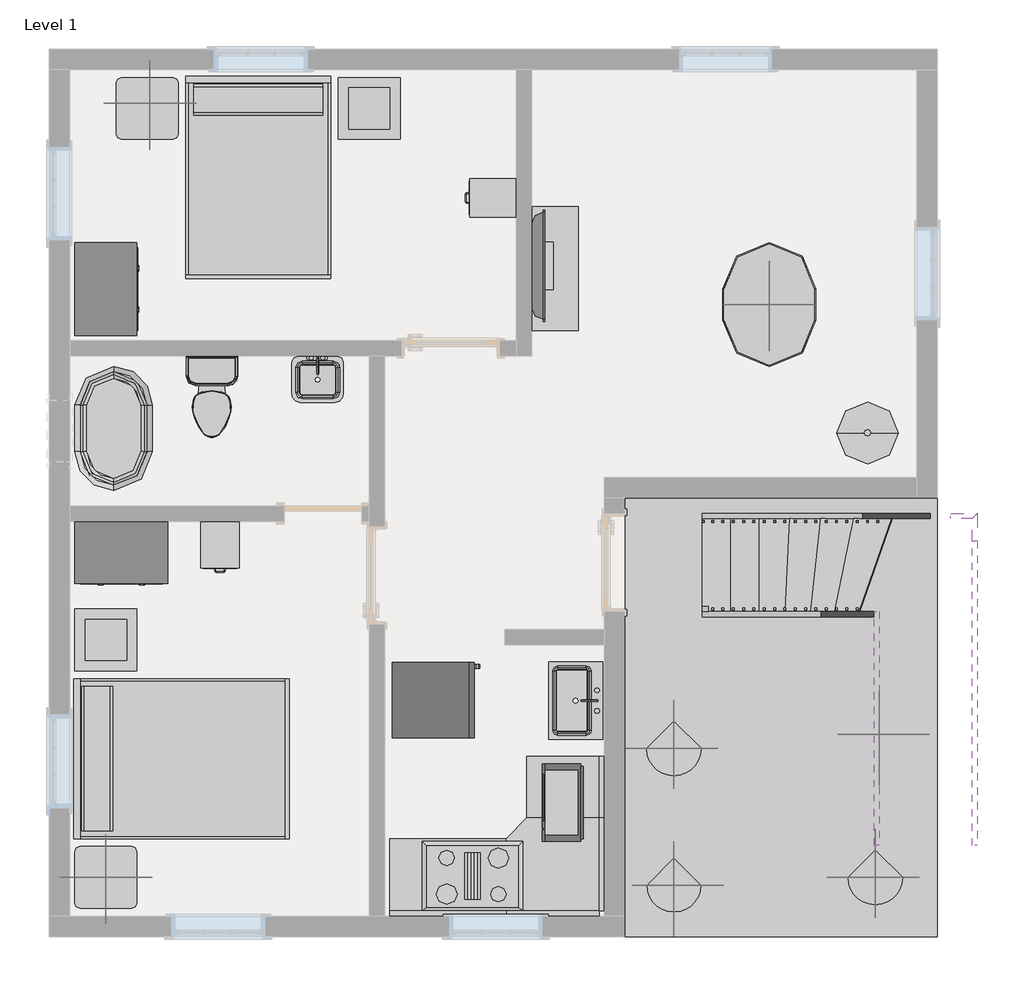
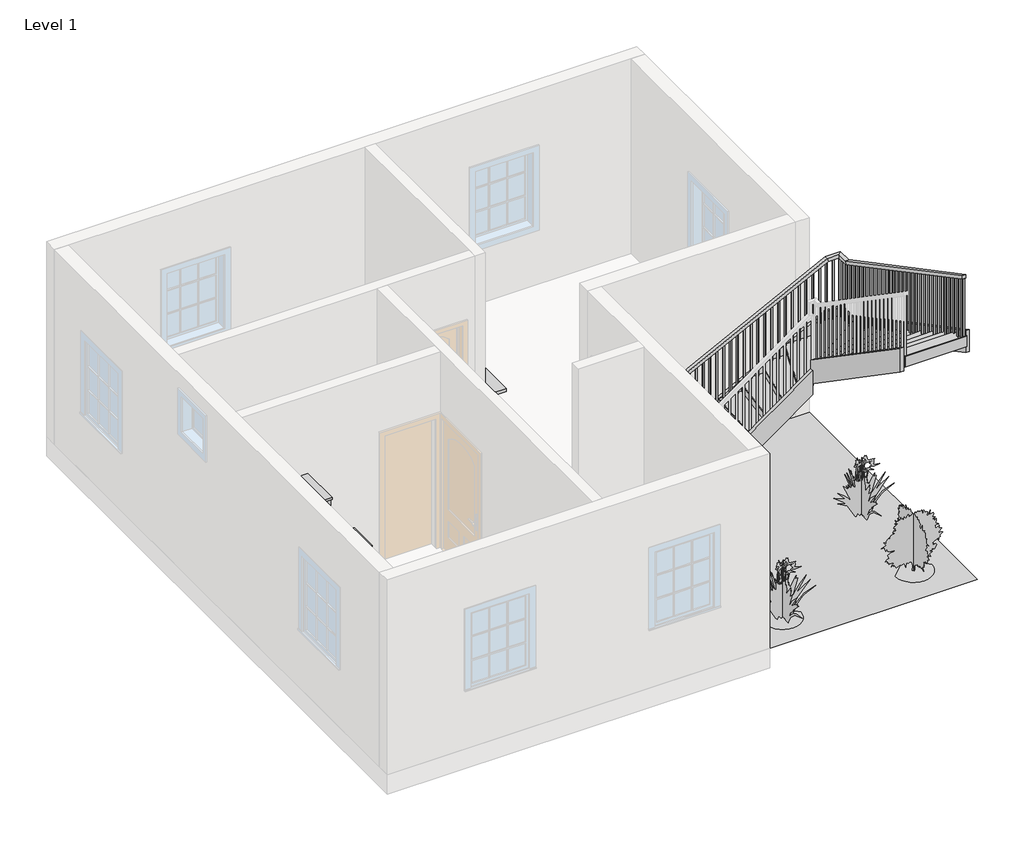
# One storey, part 2 of 2: 15 furniture elements, 7 geographic elements, 6 members, 5 flow terminals, 4 proxies, 1 railing, 1 stair flight.
"""IFC4 building model written with IfcOpenShell, lengths in millimetres."""

from ifc_helpers import new_model, si_unit, frame, origin, place, context, project, spatial, polyline, outline, extrude, faceted_brep, triangles, transform, mapped, element, save
from components import proxy_bb1e6e30, proxy_8a8d5ab2, proxy_a13a33b2, flow_terminal_accce45a, flow_terminal_38af2918, flow_terminal_62a433f7, toilet_domestic_3d_toilet_domestic_3d_f7549cf7, toilet_domestic_3d_toilet_domestic_3d_183bbd19, flow_terminal_04541809, furniture_096e7f55, furniture_35c09872, furniture_bb55ed6b, furniture_33655958, furniture_7a3aaa4f, furniture_b5c51a22, furniture_be1c6672, furniture_31d08a24, furniture_c21ab0ed, furniture_3250926c, furniture_e2d07697, rpc_plant_tropical_55f6ff97, rpc_plant_tropical_agave_1_5_93a2a214, rpc_plant_tropical_jungle_flame_3_9c4808c2, stair_flight_bb54b32b

model = new_model("IFC4")

# Units and contexts
model_context = context("Model", 3, world=origin())
ifc_project = project(units=[si_unit("LENGTHUNIT", "METRE", prefix="MILLI")], contexts=[model_context])

# Site, building, storey
site = spatial("IfcSite", under=ifc_project)
building = spatial("IfcBuilding", under=site)
storey = spatial("IfcBuildingStorey", under=building, Name="Level 1", Elevation=0.0)

# Proxies
placement = place(None, origin())
element("IfcBuildingElementProxy", 1, Name="Building Element Proxy", at=placement, inside=storey, context=model_context, shape_type="Tessellation", body=[
    triangles([(-7688.07724, 10762.3523804, 0.0), (-7688.07724, 6444.3525742, 0.0), (-4614.6770462, 6444.3525742, 0.0), (-4614.6770462, 10762.3523804, 0.0), (-7789.6768524, 6444.3525742, 0.0), (-7910.2003098, 6444.3525742, 0.0)], [[6, 5, 1], [2, 4, 1], [1, 5, 2], [2, 3, 4]], closed=False),
])
proxy_shape = proxy_bb1e6e30(model_context)
element("IfcBuildingElementProxy", 2, Name="Cook Top-4 Unit : 36\" x 20\"", ObjectType="Cook Top-4 Unit : 36\" x 20\"", at=placement, inside=storey, context=model_context, shape_type="MappedRepresentation", body=[
    mapped(proxy_shape, transform((-9186.6770189, 7041.2523405, 0.0), x_axis=(1.0, 0.0, 0.0), y_axis=(0.0, 1.0, 0.0), z_axis=(0.0, 0.0, 1.0))),
])
proxy_2_shape = proxy_8a8d5ab2(model_context)
element("IfcBuildingElementProxy", 3, Name="Microwave : 30\" x 16\" x 18\"", ObjectType="Microwave : 30\" x 16\" x 18\"", at=placement, inside=storey, context=model_context, shape_type="MappedRepresentation", body=[
    mapped(proxy_2_shape, transform((-7944.5965131, 8265.4452178, 0.0), x_axis=(0.0, -1.0000000000000002, 0.0), y_axis=(1.0000000000000002, 0.0, 0.0), z_axis=(0.0, 0.0, 1.0))),
])
proxy_3_shape = proxy_a13a33b2(model_context)
element("IfcBuildingElementProxy", 4, Name="Refrigerator : 30\" x 32\" RH", ObjectType="Refrigerator : 30\" x 32\" RH", at=placement, inside=storey, context=model_context, shape_type="MappedRepresentation", body=[
    mapped(proxy_3_shape, transform((-9585.5280474, 8773.2148405, 0.0), x_axis=(0.0, 1.0, 0.0), y_axis=(-1.0, 0.0, 0.0), z_axis=(0.0, 0.0, 1.0))),
])

# Flow terminals
flow_terminal_shape = flow_terminal_accce45a(model_context)
element("IfcFlowTerminal", 5, ObjectType="Floor Drain - Round : 5\" Strainer - 2\" Drain", at=placement, inside=storey, context=model_context, shape_type="MappedRepresentation", body=[
    mapped(flow_terminal_shape, transform((-12031.4770189, 10965.5523405, 0.0), x_axis=(1.0, 0.0, 0.0), y_axis=(0.0, 1.0, 0.0), z_axis=(0.0, 0.0, 1.0))),
])
flow_terminal_2_shape = flow_terminal_38af2918(model_context)
element("IfcFlowTerminal", 6, ObjectType="Sink Kitchen-Single : 30\" x 21\"", at=placement, inside=storey, context=model_context, shape_type="MappedRepresentation", body=[
    mapped(flow_terminal_2_shape, transform((-8173.02242, 8784.1415811, 0.0), x_axis=(0.0, -1.0000000000000004, 0.0), y_axis=(1.0000000000000004, 0.0, 0.0), z_axis=(0.0, 0.0, 1.0))),
])
flow_terminal_3_shape = flow_terminal_62a433f7(model_context)
element("IfcFlowTerminal", 7, ObjectType="Sink Vanity-Square : 20\" x 18\"", at=placement, inside=storey, context=model_context, shape_type="MappedRepresentation", body=[
    mapped(flow_terminal_3_shape, transform((-10726.3662595, 11979.2069394, 0.0), x_axis=(1.0, 0.0, 0.0), y_axis=(0.0, 1.0, 0.0), z_axis=(0.0, 0.0, 1.0))),
])
toilet_domestic_3d_toilet_domestic_3d_shape = toilet_domestic_3d_toilet_domestic_3d_f7549cf7(model_context)
toilet_domestic_3d_toilet_domestic_3d_2_shape = toilet_domestic_3d_toilet_domestic_3d_183bbd19(model_context)
element("IfcFlowTerminal", 8, ObjectType="Toilet-Domestic-3D : Toilet-Domestic-3D", at=placement, inside=storey, context=model_context, shape_type="MappedRepresentation", body=[
    mapped(toilet_domestic_3d_toilet_domestic_3d_shape, transform((-11752.0770189, 11664.6563132, 0.0), x_axis=(1.0, 0.0, 0.0), y_axis=(0.0, 1.0, 0.0), z_axis=(0.0, 0.0, 1.0))),
    mapped(toilet_domestic_3d_toilet_domestic_3d_2_shape, transform((-11752.0770189, 11664.6563132, 0.0), x_axis=(1.0, 0.0, 0.0), y_axis=(0.0, 1.0, 0.0), z_axis=(0.0, 0.0, 1.0))),
])
flow_terminal_4_shape = flow_terminal_04541809(model_context)
element("IfcFlowTerminal", 9, ObjectType="Tub-Free Standing-3D : 30\" x 60\"", at=placement, inside=storey, context=model_context, shape_type="MappedRepresentation", body=[
    mapped(flow_terminal_4_shape, transform((-12717.2770189, 11448.1523405, 0.0), x_axis=(1.0000000000000007, 0.0, 0.0), y_axis=(0.0, 1.0000000000000007, 0.0), z_axis=(0.0, 0.0, 1.0))),
])

# Furniture
furniture_shape = furniture_096e7f55(model_context)
element("IfcFurniture", 10, ObjectType="Bed-Shaker : Double 56\" x 78\"", at=placement, inside=storey, context=model_context, shape_type="MappedRepresentation", body=[
    mapped(furniture_shape, transform((-11275.8270189, 14902.5523405, 0.0), x_axis=(1.0, 0.0, 0.0), y_axis=(0.0, 1.0, 0.0), z_axis=(0.0, 0.0, 1.0))),
])
furniture_2_shape = furniture_35c09872(model_context)
element("IfcFurniture", 11, ObjectType="Bed-Shaker : Queen 62\" x 83\"", at=placement, inside=storey, context=model_context, shape_type="MappedRepresentation", body=[
    mapped(furniture_2_shape, transform((-13098.2770189, 8216.0023405, 0.0), x_axis=(0.0, 1.0, 0.0), y_axis=(-1.0, 0.0, 0.0), z_axis=(0.0, 0.0, 1.0))),
])
furniture_3_shape = furniture_bb55ed6b(model_context)
element("IfcFurniture", 12, ObjectType="Cabinet-File 2 Drawer : 15\" x 18\"", at=placement, inside=storey, context=model_context, shape_type="MappedRepresentation", body=[
    mapped(furniture_3_shape, transform((-8841.3427188, 13588.3042775, 0.0), x_axis=(0.0, -1.0000000000000004, 0.0), y_axis=(1.0000000000000004, 0.0, 0.0), z_axis=(0.0, 0.0, 1.0))),
])
element("IfcFurniture", 13, ObjectType="Cabinet-File 2 Drawer : 15\" x 18\"", at=placement, inside=storey, context=model_context, shape_type="MappedRepresentation", body=[
    mapped(furniture_3_shape, transform((-11543.5637717, 10447.2866406, 0.0), x_axis=(1.0, 0.0, 0.0), y_axis=(0.0, 1.0, 0.0), z_axis=(0.0, 0.0, 1.0))),
])
furniture_4_shape = furniture_33655958(model_context)
element("IfcFurniture", 14, ObjectType="Dresser : 48\" x 72\" x 24\"", at=placement, inside=storey, context=model_context, shape_type="MappedRepresentation", body=[
    mapped(furniture_4_shape, transform((-13156.639973, 13088.9456003, 0.0), x_axis=(0.0, 1.0000000000000002, 0.0), y_axis=(-1.0000000000000002, 0.0, 0.0), z_axis=(0.0, 0.0, 1.0))),
])
element("IfcFurniture", 15, ObjectType="Dresser : 48\" x 72\" x 24\"", at=placement, inside=storey, context=model_context, shape_type="MappedRepresentation", body=[
    mapped(furniture_4_shape, transform((-12371.8837591, 10592.1152946, 0.0), x_axis=(1.0, 0.0, 0.0), y_axis=(0.0, 1.0, 0.0), z_axis=(0.0, 0.0, 1.0))),
])
furniture_5_shape = furniture_7a3aaa4f(model_context)
element("IfcFurniture", 16, ObjectType="TV - Flat Screen : 42\"", at=placement, inside=storey, context=model_context, shape_type="MappedRepresentation", body=[
    mapped(furniture_5_shape, transform((-8543.9383953, 13052.2968547, 1041.4), x_axis=(0.0, 1.0, 0.0), y_axis=(-1.0, 0.0, 0.0), z_axis=(0.0, 0.0, 1.0))),
])
furniture_6_shape = furniture_b5c51a22(model_context)
element("IfcFurniture", 17, ObjectType="Table-Coffee : 24\" x 24\" x 24\"", at=placement, inside=storey, context=model_context, shape_type="MappedRepresentation", body=[
    mapped(furniture_6_shape, transform((-10220.9427856, 14502.5412627, 0.0), x_axis=(1.0, 0.0, 0.0), y_axis=(0.0, 1.0, 0.0), z_axis=(0.0, 0.0, 1.0))),
])
element("IfcFurniture", 18, ObjectType="Table-Coffee : 24\" x 24\" x 24\"", at=placement, inside=storey, context=model_context, shape_type="MappedRepresentation", body=[
    mapped(furniture_6_shape, transform((-12811.7427856, 9270.1412627, 0.0), x_axis=(1.0, 0.0, 0.0), y_axis=(0.0, 1.0, 0.0), z_axis=(0.0, 0.0, 1.0))),
])
furniture_7_shape = furniture_be1c6672(model_context)
element("IfcFurniture", 19, ObjectType="Table-Dining Oval : 36\" x 48\"", at=placement, inside=storey, context=model_context, shape_type="MappedRepresentation", body=[
    mapped(furniture_7_shape, transform((-6623.7753796, 13069.1720126, 0.0), x_axis=(0.0, 1.0, 0.0), y_axis=(-1.0, 0.0, 0.0), z_axis=(0.0, 0.0, 1.0))),
])
furniture_8_shape = furniture_31d08a24(model_context)
element("IfcFurniture", 20, ObjectType="Table-End : 24\" x 24\"", at=placement, inside=storey, context=model_context, shape_type="MappedRepresentation", body=[
    mapped(furniture_8_shape, transform((-12695.6106492, 14445.3523405, 0.0), x_axis=(1.0, 0.0, 0.0), y_axis=(0.0, 1.0, 0.0), z_axis=(0.0, 0.0, 1.0))),
])
element("IfcFurniture", 21, ObjectType="Table-End : 24\" x 24\"", at=placement, inside=storey, context=model_context, shape_type="MappedRepresentation", body=[
    mapped(furniture_8_shape, transform((-13102.0106492, 6876.1523405, 0.0), x_axis=(1.0, 0.0, 0.0), y_axis=(0.0, 1.0, 0.0), z_axis=(0.0, 0.0, 1.0))),
])
furniture_9_shape = furniture_c21ab0ed(model_context)
element("IfcFurniture", 22, ObjectType="Table-Rectangular : 72\" x 30\"", at=placement, inside=storey, context=model_context, shape_type="MappedRepresentation", body=[
    mapped(furniture_9_shape, transform((-8373.8770189, 13022.9523405, 0.0), x_axis=(0.0, 1.0000000000000002, 0.0), y_axis=(-1.0000000000000002, 0.0, 0.0), z_axis=(0.0, 0.0, 1.0))),
])
furniture_10_shape = furniture_3250926c(model_context)
element("IfcFurniture", 23, ObjectType="Table-Round : 36\" Diameter", at=placement, inside=storey, context=model_context, shape_type="MappedRepresentation", body=[
    mapped(furniture_10_shape, transform((-5300.4770189, 11403.7023405, 0.0), x_axis=(1.0, 0.0, 0.0), y_axis=(0.0, 1.0, 0.0), z_axis=(0.0, 0.0, 1.0))),
])
furniture_11_shape = furniture_e2d07697(model_context)
element("IfcFurniture", 24, ObjectType="Work Station Cubicle : 96\" x 96\"", at=placement, inside=storey, context=model_context, shape_type="MappedRepresentation", body=[
    mapped(furniture_11_shape, transform((-8023.0087712, 6152.5293329, 0.0), x_axis=(-1.0000000000000004, 0.0, 0.0), y_axis=(0.0, -1.0000000000000004, 0.0), z_axis=(0.0, 0.0, 1.0))),
])

# Geographic elements
rpc_plant_tropical_shape = rpc_plant_tropical_55f6ff97(model_context)
element("IfcGeographicElement", 25, ObjectType="RPC Plant - Tropical", at=placement, inside=storey, context=model_context, shape_type="MappedRepresentation", body=[
    mapped(rpc_plant_tropical_shape, transform((-7205.4770189, 6952.3523405, 0.0), x_axis=(1.0, 0.0, 0.0), y_axis=(0.0, 1.0, 0.0), z_axis=(0.0, 0.0, 1.0))),
])
element("IfcGeographicElement", 26, ObjectType="RPC Plant - Tropical", at=placement, inside=storey, context=model_context, shape_type="MappedRepresentation", body=[
    mapped(rpc_plant_tropical_shape, transform((-5183.9400294, 8435.9794452, 0.0), x_axis=(1.0, 0.0, 0.0), y_axis=(0.0, 1.0, 0.0), z_axis=(0.0, 0.0, 1.0))),
])
rpc_plant_tropical_agave_1_5_shape = rpc_plant_tropical_agave_1_5_93a2a214(model_context)
element("IfcGeographicElement", 27, ObjectType="RPC Plant - Tropical : Agave - 1.5'", at=placement, inside=storey, context=model_context, shape_type="MappedRepresentation", body=[
    mapped(rpc_plant_tropical_agave_1_5_shape, transform((-12361.6770189, 14648.5523405, 609.6), x_axis=(1.0, 0.0, 0.0), y_axis=(0.0, 1.0, 0.0), z_axis=(0.0, 0.0, 1.0))),
])
element("IfcGeographicElement", 28, ObjectType="RPC Plant - Tropical : Agave - 1.5'", at=placement, inside=storey, context=model_context, shape_type="MappedRepresentation", body=[
    mapped(rpc_plant_tropical_agave_1_5_shape, transform((-12793.4770189, 7028.5523405, 609.6), x_axis=(1.0, 0.0, 0.0), y_axis=(0.0, 1.0, 0.0), z_axis=(0.0, 0.0, 1.0))),
])
element("IfcGeographicElement", 29, ObjectType="RPC Plant - Tropical : Agave - 1.5'", at=placement, inside=storey, context=model_context, shape_type="MappedRepresentation", body=[
    mapped(rpc_plant_tropical_agave_1_5_shape, transform((-6265.6770189, 12667.3523405, 736.6), x_axis=(1.0, 0.0, 0.0), y_axis=(0.0, 1.0, 0.0), z_axis=(0.0, 0.0, 1.0))),
])
rpc_plant_tropical_jungle_flame_3_shape = rpc_plant_tropical_jungle_flame_3_9c4808c2(model_context)
element("IfcGeographicElement", 30, ObjectType="RPC Plant - Tropical : Jungle Flame - 3'", at=placement, inside=storey, context=model_context, shape_type="MappedRepresentation", body=[
    mapped(rpc_plant_tropical_jungle_flame_3_shape, transform((-5224.2770189, 7028.5523405, 0.0), x_axis=(1.0, 0.0, 0.0), y_axis=(0.0, 1.0, 0.0), z_axis=(0.0, 0.0, 1.0))),
])
element("IfcGeographicElement", 31, ObjectType="RPC Plant - Tropical : Jungle Flame - 3'", at=placement, inside=storey, context=model_context, shape_type="MappedRepresentation", body=[
    mapped(rpc_plant_tropical_jungle_flame_3_shape, transform((-7205.4770189, 8298.5523405, 0.0), x_axis=(1.0, 0.0, 0.0), y_axis=(0.0, 1.0, 0.0), z_axis=(0.0, 0.0, 1.0))),
])

# Members
element("IfcMember", 32, ObjectType="Stringer - 2\" Width", at=placement, inside=storey, context=model_context, shape_type="SweptSolid", body=[
    extrude(outline(polyline([(400.2693042, -6926.0770189), (58.2694253, -6926.0770189), (1301.1254742, -4483.8835542), (1643.1253532, -4483.8835542), (400.2693042, -6926.0770189)])), frame((0.0, 10559.1523405, 0.0), z_axis=(0.0, 1.0, 0.0), x_axis=(0.0, 0.0, 1.0)), (0.0, 0.0, 1.0), 50.8),
])
element("IfcMember", 33, ObjectType="Stringer - 2\" Width", at=placement, inside=storey, context=model_context, shape_type="SweptSolid", body=[
    extrude(outline(polyline([(-4483.8835542, 10559.1523405), (-4483.8835542, 10609.9523405), (-4218.7400294, 10609.9523405), (-4269.5400294, 10559.1523405), (-4483.8835542, 10559.1523405)])), frame((0.0, 0.0, 1301.1254742), z_axis=(0.0, 0.0, 1.0), x_axis=(1.0, 0.0, 0.0)), (0.0, 0.0, 1.0), 341.9998789),
])
element("IfcMember", 34, ObjectType="Stringer - 2\" Width", at=placement, inside=storey, context=model_context, shape_type="SweptSolid", body=[
    extrude(outline(polyline([(-4269.5400294, 10559.1523405), (-4218.7400294, 10609.9523405), (-4218.7400294, 10338.1416337), (-4269.5400294, 10338.1416337), (-4269.5400294, 10559.1523405)])), frame((0.0, 0.0, 1301.1254742), z_axis=(0.0, 0.0, 1.0), x_axis=(1.0, 0.0, 0.0)), (0.0, 0.0, 1.0), 341.9998789),
])
element("IfcMember", 35, ObjectType="Stringer - 2\" Width", at=placement, inside=storey, context=model_context, shape_type="SweptSolid", body=[
    extrude(outline(polyline([(10338.1416337, 1643.1253532), (10338.1416337, 1301.1254742), (7343.815351, 2888.5842782), (7343.815351, 3230.5841571), (10338.1416337, 1643.1253532)])), frame((-4269.5400294, 0.0, 0.0), z_axis=(1.0, 0.0, 0.0), x_axis=(0.0, 1.0, 0.0)), (0.0, 0.0, 1.0), 50.8),
])
element("IfcMember", 36, ObjectType="Stringer - 2\" Width", at=placement, inside=storey, context=model_context, shape_type="SweptSolid", body=[
    extrude(outline(polyline([(361.2386526, -6926.0770189), (0.0, -6926.0770189), (0.0, -6906.2317896), (1202.8652744, -5234.7400294), (1578.385264, -5234.7400294), (361.2386526, -6926.0770189)])), frame((0.0, 9593.9523405, 0.0), z_axis=(0.0, 1.0, 0.0), x_axis=(0.0, 0.0, 1.0)), (0.0, 0.0, 1.0), 50.8),
])
element("IfcMember", 37, ObjectType="Stringer - 2\" Width", at=placement, inside=storey, context=model_context, shape_type="SweptSolid", body=[
    extrude(outline(polyline([(9644.7523405, 1709.1912062), (9644.7523405, 1339.3192248), (7343.815351, 2921.0520077), (7343.815351, 3290.9239891), (9644.7523405, 1709.1912062)])), frame((-5234.7400294, 0.0, 0.0), z_axis=(1.0, 0.0, 0.0), x_axis=(0.0, 1.0, 0.0)), (0.0, 0.0, 1.0), 50.8),
])

# Railing
element("IfcRailing", 38, ObjectType="Handrail - Rectangular", at=placement, inside=storey, context=model_context, shape_type="SolidModel", body=[
    faceted_brep([(-6926.0770189, 10559.1523405, 1280.2106178), (-6926.0770189, 10559.1523405, 1223.2106379), (-6926.0770189, 10508.3523405, 1223.2106379), (-6926.0770189, 10508.3523405, 1280.2106178), (-4491.3002998, 10559.1523405, 2519.2922126), (-4479.1174326, 10559.1523405, 2468.4922126), (-4479.1174326, 10508.3523405, 2468.4922126), (-4491.3002998, 10508.3523405, 2519.2922126), (-4269.5400294, 10559.1523405, 2519.2922126), (-4269.5400294, 10559.1523405, 2468.4922126), (-4320.3400294, 10508.3523405, 2468.4922126), (-4320.3400294, 10508.3523405, 2519.2922126), (-4269.5400294, 10345.2611552, 2519.2922126), (-4269.5400294, 10332.6279903, 2468.4922126), (-4320.3400294, 10332.6279903, 2468.4922126), (-4320.3400294, 10345.2611552, 2519.2922126), (-4269.5400294, 7343.815351, 4110.5254706), (-4320.3400294, 7343.815351, 4110.5254706), (-4320.3400294, 7343.815351, 4053.0279277), (-4269.5400294, 7343.815351, 4053.0279277)], [[[0, 1, 2, 3]], [[1, 0, 4, 5]], [[2, 1, 5, 6]], [[3, 2, 6, 7]], [[0, 3, 7, 4]], [[5, 4, 8, 9]], [[6, 5, 9, 10]], [[7, 6, 10, 11]], [[4, 7, 11, 8]], [[9, 8, 12, 13]], [[10, 9, 13, 14]], [[11, 10, 14, 15]], [[8, 11, 15, 12]], [[16, 17, 18, 19]], [[13, 12, 16, 19]], [[14, 13, 19, 18]], [[15, 14, 18, 17]], [[12, 15, 17, 16]]]),
    extrude(outline(polyline([(7408.3861552, 4018.7953552), (7408.3861552, 3048.0), (7389.3361552, 3048.0), (7389.3361552, 4028.8948191), (7408.3861552, 4018.7953552)])), frame((-4304.4650294, 0.0, 0.0), z_axis=(1.0, 0.0, 0.0), x_axis=(0.0, 1.0, 0.0)), (0.0, 0.0, 1.0), 19.05),
    extrude(outline(polyline([(7509.9861552, 3964.9315477), (7509.9861552, 3048.0), (7490.9361552, 3048.0), (7490.9361552, 3975.0310116), (7509.9861552, 3964.9315477)])), frame((-4304.4650294, 0.0, 0.0), z_axis=(1.0, 0.0, 0.0), x_axis=(0.0, 1.0, 0.0)), (0.0, 0.0, 1.0), 19.05),
    extrude(outline(polyline([(7611.5861552, 3911.0677402), (7611.5861552, 3048.0), (7592.5361552, 3048.0), (7592.5361552, 3921.1672041), (7611.5861552, 3911.0677402)])), frame((-4304.4650294, 0.0, 0.0), z_axis=(1.0, 0.0, 0.0), x_axis=(0.0, 1.0, 0.0)), (0.0, 0.0, 1.0), 19.05),
    extrude(outline(polyline([(7713.1861552, 3857.2039327), (7713.1861552, 2878.6666667), (7694.1361552, 2878.6666667), (7694.1361552, 3867.3033966), (7713.1861552, 3857.2039327)])), frame((-4304.4650294, 0.0, 0.0), z_axis=(1.0, 0.0, 0.0), x_axis=(0.0, 1.0, 0.0)), (0.0, 0.0, 1.0), 19.05),
    extrude(outline(polyline([(7814.7861552, 3803.3401252), (7814.7861552, 2878.6666667), (7795.7361552, 2878.6666667), (7795.7361552, 3813.4395891), (7814.7861552, 3803.3401252)])), frame((-4304.4650294, 0.0, 0.0), z_axis=(1.0, 0.0, 0.0), x_axis=(0.0, 1.0, 0.0)), (0.0, 0.0, 1.0), 19.05),
    extrude(outline(polyline([(7916.3861552, 3749.4763177), (7916.3861552, 2709.3333333), (7897.3361552, 2709.3333333), (7897.3361552, 3759.5757816), (7916.3861552, 3749.4763177)])), frame((-4304.4650294, 0.0, 0.0), z_axis=(1.0, 0.0, 0.0), x_axis=(0.0, 1.0, 0.0)), (0.0, 0.0, 1.0), 19.05),
    extrude(outline(polyline([(8017.9861552, 3695.6125102), (8017.9861552, 2709.3333333), (7998.9361552, 2709.3333333), (7998.9361552, 3705.7119741), (8017.9861552, 3695.6125102)])), frame((-4304.4650294, 0.0, 0.0), z_axis=(1.0, 0.0, 0.0), x_axis=(0.0, 1.0, 0.0)), (0.0, 0.0, 1.0), 19.05),
    extrude(outline(polyline([(8119.5861552, 3641.7487027), (8119.5861552, 2709.3333333), (8100.5361552, 2709.3333333), (8100.5361552, 3651.8481666), (8119.5861552, 3641.7487027)])), frame((-4304.4650294, 0.0, 0.0), z_axis=(1.0, 0.0, 0.0), x_axis=(0.0, 1.0, 0.0)), (0.0, 0.0, 1.0), 19.05),
    extrude(outline(polyline([(8221.1861552, 3587.8848952), (8221.1861552, 2540.0), (8202.1361552, 2540.0), (8202.1361552, 3597.9843591), (8221.1861552, 3587.8848952)])), frame((-4304.4650294, 0.0, 0.0), z_axis=(1.0, 0.0, 0.0), x_axis=(0.0, 1.0, 0.0)), (0.0, 0.0, 1.0), 19.05),
    extrude(outline(polyline([(8322.7861552, 3534.0210877), (8322.7861552, 2540.0), (8303.7361552, 2540.0), (8303.7361552, 3544.1205516), (8322.7861552, 3534.0210877)])), frame((-4304.4650294, 0.0, 0.0), z_axis=(1.0, 0.0, 0.0), x_axis=(0.0, 1.0, 0.0)), (0.0, 0.0, 1.0), 19.05),
    extrude(outline(polyline([(8424.3861552, 3480.1572802), (8424.3861552, 2540.0), (8405.3361552, 2540.0), (8405.3361552, 3490.2567441), (8424.3861552, 3480.1572802)])), frame((-4304.4650294, 0.0, 0.0), z_axis=(1.0, 0.0, 0.0), x_axis=(0.0, 1.0, 0.0)), (0.0, 0.0, 1.0), 19.05),
    extrude(outline(polyline([(8525.9861552, 3426.2934727), (8525.9861552, 2370.6666667), (8506.9361552, 2370.6666667), (8506.9361552, 3436.3929366), (8525.9861552, 3426.2934727)])), frame((-4304.4650294, 0.0, 0.0), z_axis=(1.0, 0.0, 0.0), x_axis=(0.0, 1.0, 0.0)), (0.0, 0.0, 1.0), 19.05),
    extrude(outline(polyline([(8627.5861552, 3372.4296652), (8627.5861552, 2370.6666667), (8608.5361552, 2370.6666667), (8608.5361552, 3382.5291291), (8627.5861552, 3372.4296652)])), frame((-4304.4650294, 0.0, 0.0), z_axis=(1.0, 0.0, 0.0), x_axis=(0.0, 1.0, 0.0)), (0.0, 0.0, 1.0), 19.05),
    extrude(outline(polyline([(8729.1861552, 3318.5658577), (8729.1861552, 2370.6666667), (8710.1361552, 2370.6666667), (8710.1361552, 3328.6653216), (8729.1861552, 3318.5658577)])), frame((-4304.4650294, 0.0, 0.0), z_axis=(1.0, 0.0, 0.0), x_axis=(0.0, 1.0, 0.0)), (0.0, 0.0, 1.0), 19.05),
    extrude(outline(polyline([(8830.7861552, 3264.7020502), (8830.7861552, 2201.3333333), (8811.7361552, 2201.3333333), (8811.7361552, 3274.8015141), (8830.7861552, 3264.7020502)])), frame((-4304.4650294, 0.0, 0.0), z_axis=(1.0, 0.0, 0.0), x_axis=(0.0, 1.0, 0.0)), (0.0, 0.0, 1.0), 19.05),
    extrude(outline(polyline([(8932.3861552, 3210.8382427), (8932.3861552, 2201.3333333), (8913.3361552, 2201.3333333), (8913.3361552, 3220.9377066), (8932.3861552, 3210.8382427)])), frame((-4304.4650294, 0.0, 0.0), z_axis=(1.0, 0.0, 0.0), x_axis=(0.0, 1.0, 0.0)), (0.0, 0.0, 1.0), 19.05),
    extrude(outline(polyline([(9033.9861552, 3156.9744352), (9033.9861552, 2201.3333333), (9014.9361552, 2201.3333333), (9014.9361552, 3167.0738991), (9033.9861552, 3156.9744352)])), frame((-4304.4650294, 0.0, 0.0), z_axis=(1.0, 0.0, 0.0), x_axis=(0.0, 1.0, 0.0)), (0.0, 0.0, 1.0), 19.05),
    extrude(outline(polyline([(9135.5861552, 3103.1106277), (9135.5861552, 2032.0), (9116.5361552, 2032.0), (9116.5361552, 3113.2100916), (9135.5861552, 3103.1106277)])), frame((-4304.4650294, 0.0, 0.0), z_axis=(1.0, 0.0, 0.0), x_axis=(0.0, 1.0, 0.0)), (0.0, 0.0, 1.0), 19.05),
    extrude(outline(polyline([(9237.1861552, 3049.2468202), (9237.1861552, 2032.0), (9218.1361552, 2032.0), (9218.1361552, 3059.3462841), (9237.1861552, 3049.2468202)])), frame((-4304.4650294, 0.0, 0.0), z_axis=(1.0, 0.0, 0.0), x_axis=(0.0, 1.0, 0.0)), (0.0, 0.0, 1.0), 19.05),
    extrude(outline(polyline([(9338.7861552, 2995.3830127), (9338.7861552, 2032.0), (9319.7361552, 2032.0), (9319.7361552, 3005.4824766), (9338.7861552, 2995.3830127)])), frame((-4304.4650294, 0.0, 0.0), z_axis=(1.0, 0.0, 0.0), x_axis=(0.0, 1.0, 0.0)), (0.0, 0.0, 1.0), 19.05),
    extrude(outline(polyline([(9440.3861552, 2941.5192052), (9440.3861552, 1862.6666667), (9421.3361552, 1862.6666667), (9421.3361552, 2951.6186691), (9440.3861552, 2941.5192052)])), frame((-4304.4650294, 0.0, 0.0), z_axis=(1.0, 0.0, 0.0), x_axis=(0.0, 1.0, 0.0)), (0.0, 0.0, 1.0), 19.05),
    extrude(outline(polyline([(9541.9861552, 2887.6553977), (9541.9861552, 1862.6666667), (9522.9361552, 1862.6666667), (9522.9361552, 2897.7548616), (9541.9861552, 2887.6553977)])), frame((-4304.4650294, 0.0, 0.0), z_axis=(1.0, 0.0, 0.0), x_axis=(0.0, 1.0, 0.0)), (0.0, 0.0, 1.0), 19.05),
    extrude(outline(polyline([(9643.5861552, 2833.7915902), (9643.5861552, 1862.6666667), (9624.5361552, 1862.6666667), (9624.5361552, 2843.8910541), (9643.5861552, 2833.7915902)])), frame((-4304.4650294, 0.0, 0.0), z_axis=(1.0, 0.0, 0.0), x_axis=(0.0, 1.0, 0.0)), (0.0, 0.0, 1.0), 19.05),
    extrude(outline(polyline([(9745.1861552, 2779.9277827), (9745.1861552, 1862.6666667), (9726.1361552, 1862.6666667), (9726.1361552, 2790.0272466), (9745.1861552, 2779.9277827)])), frame((-4304.4650294, 0.0, 0.0), z_axis=(1.0, 0.0, 0.0), x_axis=(0.0, 1.0, 0.0)), (0.0, 0.0, 1.0), 19.05),
    extrude(outline(polyline([(9846.7861552, 2726.0639752), (9846.7861552, 1693.3333333), (9827.7361552, 1693.3333333), (9827.7361552, 2736.1634391), (9846.7861552, 2726.0639752)])), frame((-4304.4650294, 0.0, 0.0), z_axis=(1.0, 0.0, 0.0), x_axis=(0.0, 1.0, 0.0)), (0.0, 0.0, 1.0), 19.05),
    extrude(outline(polyline([(9948.3861552, 2672.2001677), (9948.3861552, 1693.3333333), (9929.3361552, 1693.3333333), (9929.3361552, 2682.2996316), (9948.3861552, 2672.2001677)])), frame((-4304.4650294, 0.0, 0.0), z_axis=(1.0, 0.0, 0.0), x_axis=(0.0, 1.0, 0.0)), (0.0, 0.0, 1.0), 19.05),
    extrude(outline(polyline([(10049.9861552, 2618.3363602), (10049.9861552, 1693.3333333), (10030.9361552, 1693.3333333), (10030.9361552, 2628.4358241), (10049.9861552, 2618.3363602)])), frame((-4304.4650294, 0.0, 0.0), z_axis=(1.0, 0.0, 0.0), x_axis=(0.0, 1.0, 0.0)), (0.0, 0.0, 1.0), 19.05),
    extrude(outline(polyline([(10151.5861552, 2564.4725527), (10151.5861552, 1693.3333333), (10132.5361552, 1693.3333333), (10132.5361552, 2574.5720166), (10151.5861552, 2564.4725527)])), frame((-4304.4650294, 0.0, 0.0), z_axis=(1.0, 0.0, 0.0), x_axis=(0.0, 1.0, 0.0)), (0.0, 0.0, 1.0), 19.05),
    extrude(outline(polyline([(10253.1861552, 2510.6087452), (10253.1861552, 1524.0), (10234.1361552, 1524.0), (10234.1361552, 2520.7082091), (10253.1861552, 2510.6087452)])), frame((-4304.4650294, 0.0, 0.0), z_axis=(1.0, 0.0, 0.0), x_axis=(0.0, 1.0, 0.0)), (0.0, 0.0, 1.0), 19.05),
    extrude(outline(polyline([(-4285.4150294, 10441.6773405), (-4285.4150294, 10422.6273405), (-4304.4650294, 10422.6273405), (-4304.4650294, 10441.6773405), (-4285.4150294, 10441.6773405)])), frame((0.0, 0.0, 1524.0), z_axis=(0.0, 0.0, 1.0), x_axis=(1.0, 0.0, 0.0)), (0.0, 0.0, 1.0), 944.4922126),
    extrude(outline(polyline([(-4399.2252998, 10543.2773405), (-4380.1752998, 10543.2773405), (-4380.1752998, 10524.2273405), (-4399.2252998, 10524.2273405), (-4399.2252998, 10543.2773405)])), frame((0.0, 0.0, 1524.0), z_axis=(0.0, 0.0, 1.0), x_axis=(1.0, 0.0, 0.0)), (0.0, 0.0, 1.0), 944.4922126),
    extrude(outline(polyline([(2407.5835605, -4598.8020189), (1524.0, -4598.8020189), (1524.0, -4579.7520189), (2417.2782911, -4579.7520189), (2407.5835605, -4598.8020189)])), frame((0.0, 10524.2273405, 0.0), z_axis=(0.0, 1.0, 0.0), x_axis=(0.0, 0.0, 1.0)), (0.0, 0.0, 1.0), 19.05),
    extrude(outline(polyline([(2355.8783306, -4700.4020189), (1354.6666667, -4700.4020189), (1354.6666667, -4681.3520189), (2365.5730612, -4681.3520189), (2355.8783306, -4700.4020189)])), frame((0.0, 10524.2273405, 0.0), z_axis=(0.0, 1.0, 0.0), x_axis=(0.0, 0.0, 1.0)), (0.0, 0.0, 1.0), 19.05),
    extrude(outline(polyline([(2304.1731007, -4802.0020189), (1354.6666667, -4802.0020189), (1354.6666667, -4782.9520189), (2313.8678313, -4782.9520189), (2304.1731007, -4802.0020189)])), frame((0.0, 10524.2273405, 0.0), z_axis=(0.0, 1.0, 0.0), x_axis=(0.0, 0.0, 1.0)), (0.0, 0.0, 1.0), 19.05),
    extrude(outline(polyline([(2252.4678708, -4903.6020189), (1354.6666667, -4903.6020189), (1354.6666667, -4884.5520189), (2262.1626014, -4884.5520189), (2252.4678708, -4903.6020189)])), frame((0.0, 10524.2273405, 0.0), z_axis=(0.0, 1.0, 0.0), x_axis=(0.0, 0.0, 1.0)), (0.0, 0.0, 1.0), 19.05),
    extrude(outline(polyline([(2200.7626409, -5005.2020189), (1354.6666667, -5005.2020189), (1354.6666667, -4986.1520189), (2210.4573715, -4986.1520189), (2200.7626409, -5005.2020189)])), frame((0.0, 10524.2273405, 0.0), z_axis=(0.0, 1.0, 0.0), x_axis=(0.0, 0.0, 1.0)), (0.0, 0.0, 1.0), 19.05),
    extrude(outline(polyline([(2149.0574109, -5106.8020189), (1354.6666667, -5106.8020189), (1354.6666667, -5087.7520189), (2158.7521416, -5087.7520189), (2149.0574109, -5106.8020189)])), frame((0.0, 10524.2273405, 0.0), z_axis=(0.0, 1.0, 0.0), x_axis=(0.0, 0.0, 1.0)), (0.0, 0.0, 1.0), 19.05),
    extrude(outline(polyline([(2097.352181, -5208.4020189), (1185.3333333, -5208.4020189), (1185.3333333, -5189.3520189), (2107.0469116, -5189.3520189), (2097.352181, -5208.4020189)])), frame((0.0, 10524.2273405, 0.0), z_axis=(0.0, 1.0, 0.0), x_axis=(0.0, 0.0, 1.0)), (0.0, 0.0, 1.0), 19.05),
    extrude(outline(polyline([(2045.6469511, -5310.0020189), (1185.3333333, -5310.0020189), (1185.3333333, -5290.9520189), (2055.3416817, -5290.9520189), (2045.6469511, -5310.0020189)])), frame((0.0, 10524.2273405, 0.0), z_axis=(0.0, 1.0, 0.0), x_axis=(0.0, 0.0, 1.0)), (0.0, 0.0, 1.0), 19.05),
    extrude(outline(polyline([(1993.9417212, -5411.6020189), (1185.3333333, -5411.6020189), (1185.3333333, -5392.5520189), (2003.6364518, -5392.5520189), (1993.9417212, -5411.6020189)])), frame((0.0, 10524.2273405, 0.0), z_axis=(0.0, 1.0, 0.0), x_axis=(0.0, 0.0, 1.0)), (0.0, 0.0, 1.0), 19.05),
    extrude(outline(polyline([(1942.2364913, -5513.2020189), (1016.0, -5513.2020189), (1016.0, -5494.1520189), (1951.9312219, -5494.1520189), (1942.2364913, -5513.2020189)])), frame((0.0, 10524.2273405, 0.0), z_axis=(0.0, 1.0, 0.0), x_axis=(0.0, 0.0, 1.0)), (0.0, 0.0, 1.0), 19.05),
    extrude(outline(polyline([(1890.5312614, -5614.8020189), (1016.0, -5614.8020189), (1016.0, -5595.7520189), (1900.225992, -5595.7520189), (1890.5312614, -5614.8020189)])), frame((0.0, 10524.2273405, 0.0), z_axis=(0.0, 1.0, 0.0), x_axis=(0.0, 0.0, 1.0)), (0.0, 0.0, 1.0), 19.05),
    extrude(outline(polyline([(1838.8260315, -5716.4020189), (1016.0, -5716.4020189), (1016.0, -5697.3520189), (1848.5207621, -5697.3520189), (1838.8260315, -5716.4020189)])), frame((0.0, 10524.2273405, 0.0), z_axis=(0.0, 1.0, 0.0), x_axis=(0.0, 0.0, 1.0)), (0.0, 0.0, 1.0), 19.05),
    extrude(outline(polyline([(1787.1208016, -5818.0020189), (846.6666667, -5818.0020189), (846.6666667, -5798.9520189), (1796.8155322, -5798.9520189), (1787.1208016, -5818.0020189)])), frame((0.0, 10524.2273405, 0.0), z_axis=(0.0, 1.0, 0.0), x_axis=(0.0, 0.0, 1.0)), (0.0, 0.0, 1.0), 19.05),
    extrude(outline(polyline([(1735.4155717, -5919.6020189), (846.6666667, -5919.6020189), (846.6666667, -5900.5520189), (1745.1103023, -5900.5520189), (1735.4155717, -5919.6020189)])), frame((0.0, 10524.2273405, 0.0), z_axis=(0.0, 1.0, 0.0), x_axis=(0.0, 0.0, 1.0)), (0.0, 0.0, 1.0), 19.05),
    extrude(outline(polyline([(1683.7103418, -6021.2020189), (846.6666667, -6021.2020189), (846.6666667, -6002.1520189), (1693.4050724, -6002.1520189), (1683.7103418, -6021.2020189)])), frame((0.0, 10524.2273405, 0.0), z_axis=(0.0, 1.0, 0.0), x_axis=(0.0, 0.0, 1.0)), (0.0, 0.0, 1.0), 19.05),
    extrude(outline(polyline([(1632.0051119, -6122.8020189), (677.3333333, -6122.8020189), (677.3333333, -6103.7520189), (1641.6998425, -6103.7520189), (1632.0051119, -6122.8020189)])), frame((0.0, 10524.2273405, 0.0), z_axis=(0.0, 1.0, 0.0), x_axis=(0.0, 0.0, 1.0)), (0.0, 0.0, 1.0), 19.05),
    extrude(outline(polyline([(1580.299882, -6224.4020189), (677.3333333, -6224.4020189), (677.3333333, -6205.3520189), (1589.9946126, -6205.3520189), (1580.299882, -6224.4020189)])), frame((0.0, 10524.2273405, 0.0), z_axis=(0.0, 1.0, 0.0), x_axis=(0.0, 0.0, 1.0)), (0.0, 0.0, 1.0), 19.05),
    extrude(outline(polyline([(1528.5946521, -6326.0020189), (677.3333333, -6326.0020189), (677.3333333, -6306.9520189), (1538.2893827, -6306.9520189), (1528.5946521, -6326.0020189)])), frame((0.0, 10524.2273405, 0.0), z_axis=(0.0, 1.0, 0.0), x_axis=(0.0, 0.0, 1.0)), (0.0, 0.0, 1.0), 19.05),
    extrude(outline(polyline([(1476.8894222, -6427.6020189), (508.0, -6427.6020189), (508.0, -6408.5520189), (1486.5841528, -6408.5520189), (1476.8894222, -6427.6020189)])), frame((0.0, 10524.2273405, 0.0), z_axis=(0.0, 1.0, 0.0), x_axis=(0.0, 0.0, 1.0)), (0.0, 0.0, 1.0), 19.05),
    extrude(outline(polyline([(1425.1841923, -6529.2020189), (508.0, -6529.2020189), (508.0, -6510.1520189), (1434.8789229, -6510.1520189), (1425.1841923, -6529.2020189)])), frame((0.0, 10524.2273405, 0.0), z_axis=(0.0, 1.0, 0.0), x_axis=(0.0, 0.0, 1.0)), (0.0, 0.0, 1.0), 19.05),
    extrude(outline(polyline([(1373.4789623, -6630.8020189), (508.0, -6630.8020189), (508.0, -6611.7520189), (1383.173693, -6611.7520189), (1373.4789623, -6630.8020189)])), frame((0.0, 10524.2273405, 0.0), z_axis=(0.0, 1.0, 0.0), x_axis=(0.0, 0.0, 1.0)), (0.0, 0.0, 1.0), 19.05),
    extrude(outline(polyline([(1321.7737324, -6732.4020189), (338.6666667, -6732.4020189), (338.6666667, -6713.3520189), (1331.468463, -6713.3520189), (1321.7737324, -6732.4020189)])), frame((0.0, 10524.2273405, 0.0), z_axis=(0.0, 1.0, 0.0), x_axis=(0.0, 0.0, 1.0)), (0.0, 0.0, 1.0), 19.05),
    extrude(outline(polyline([(1270.0685025, -6834.0020189), (338.6666667, -6834.0020189), (338.6666667, -6814.9520189), (1279.7632331, -6814.9520189), (1270.0685025, -6834.0020189)])), frame((0.0, 10524.2273405, 0.0), z_axis=(0.0, 1.0, 0.0), x_axis=(0.0, 0.0, 1.0)), (0.0, 0.0, 1.0), 19.05),
    extrude(outline(polyline([(-4285.4150294, 10354.7861552), (-4285.4150294, 10335.7361552), (-4304.4650294, 10335.7361552), (-4304.4650294, 10354.7861552), (-4285.4150294, 10354.7861552)])), frame((0.0, 0.0, 1524.0), z_axis=(0.0, 0.0, 1.0), x_axis=(1.0, 0.0, 0.0)), (0.0, 0.0, 1.0), 944.4922126),
    extrude(outline(polyline([(-4304.4650294, 10543.2773405), (-4285.4150294, 10543.2773405), (-4285.4150294, 10524.2273405), (-4304.4650294, 10524.2273405), (-4304.4650294, 10543.2773405)])), frame((0.0, 0.0, 1524.0), z_axis=(0.0, 0.0, 1.0), x_axis=(1.0, 0.0, 0.0)), (0.0, 0.0, 1.0), 944.4922126),
    extrude(outline(polyline([(2457.4448675, -4500.8252998), (1524.0, -4500.8252998), (1524.0, -4481.7752998), (2467.1395981, -4481.7752998), (2457.4448675, -4500.8252998)])), frame((0.0, 10524.2273405, 0.0), z_axis=(0.0, 1.0, 0.0), x_axis=(0.0, 0.0, 1.0)), (0.0, 0.0, 1.0), 19.05),
    extrude(outline(polyline([(7362.865351, 4042.9284638), (7362.865351, 3048.0), (7343.815351, 3048.0), (7343.815351, 4053.0279277), (7362.865351, 4042.9284638)])), frame((-4304.4650294, 0.0, 0.0), z_axis=(1.0, 0.0, 0.0), x_axis=(0.0, 1.0, 0.0)), (0.0, 0.0, 1.0), 19.05),
    extrude(outline(polyline([(1223.2106379, -6926.0770189), (338.6666667, -6926.0770189), (338.6666667, -6907.0270189), (1232.9053685, -6907.0270189), (1223.2106379, -6926.0770189)])), frame((0.0, 10524.2273405, 0.0), z_axis=(0.0, 1.0, 0.0), x_axis=(0.0, 0.0, 1.0)), (0.0, 0.0, 1.0), 19.05),
])

# Stair flight
stair_flight_shape = stair_flight_bb54b32b(model_context)
element("IfcStairFlight", 39, ObjectType="2\" Tread 1\" Nosing 1/4\" Riser", at=placement, inside=storey, context=model_context, shape_type="MappedRepresentation", body=[
    mapped(stair_flight_shape, transform((0.0, 0.0, 0.0), x_axis=(1.0, 0.0, 0.0), y_axis=(0.0, 1.0, 0.0), z_axis=(0.0, 0.0, 1.0))),
])

save(model, "model.ifc")

# Revit data of these elements
# Type "Cook Top-4 Unit : 36\" x 20\""
#   Assembly Code = "E1090400"
#   Depth = 2' - 0"
#   Width = 3' - 0"
#   Burner Material = Steel, Chrome Plated
#   Cooktop Material = Steel, Polished
#   Default Elevation = 0
# Type "Microwave : 30\" x 16\" x 18\""
#   Assembly Code = "E1090400"
#   Depth = 1' - 4"
#   Height = 1' - 6"
#   Width = 2' - 6"
#   Microwave Material = Laminate, Linen, Matte
#   Default Elevation = 0
# Type "Refrigerator : 30\" x 32\" RH"
#   Label = "REF."
#   Assembly Code = "E1090400"
#   Depth = 2' - 7 3/4"
#   Handle = 2' - 3"
#   Height = 5' - 10"
#   Rear Clearance = 0' - 2"
#   Top Door Height = 1' - 8"
#   Width = 2' - 5 3/8"
#   Material = Carpet (1)
#   Default Elevation = 0
# Type "Floor Drain - Round : 5\" Strainer - 2\" Drain"
#   WFU = 2
#   Strainer Height = 0' - 3 1/4"
#   Strainer Radius = 0' - 2 1/2"
#   Strainer Diameter = 0' - 5"
#   Radius 6 = 0' - 0 5/8"
#   Radius 5 = 0' - 1 1/4"
#   Radius 4 = 0' - 1 7/8"
#   Radius 2 = 0' - 3.04167"
#   Radius 1 = 0' - 2.02083"
#   Radius 3 = 0' - 2 1/32"
#   Pipe Radius = 1"
#   Pipe Diameter = 2"
#   Height 2 = 0' - 0.725"
#   Height 1 = 0' - 1 13/16"
#   Body Radius = 0' - 4 1/16"
#   Body Height = 0' - 3 5/8"
#   Body Diameter = 0' - 8 1/8"
#   Drain Material = none
#   HWFU = 0
#   Default Elevation = 0
#   CWFU = 0
# Type "Sink Kitchen-Single : 30\" x 21\""
#   Assembly Code = "D2010410"
#   Counter Height = 3' - 0"
#   Depth = 1' - 9"
#   Width = 2' - 6"
#   Faucet Material = Steel, Polished
#   Sink Material = Steel, Polished
#   Default Elevation = 0
# Type "Sink Vanity-Square : 20\" x 18\""
#   Assembly Code = "D2010400"
#   Counter Height = 2' - 7"
#   Depth = 1' - 6"
#   Width = 1' - 8"
#   Basin Material = Porcelain, Linen
#   Faucet Material = Steel, Polished
#   Default Elevation = 0
# Type "Toilet-Domestic-3D : Toilet-Domestic-3D"
#   Assembly Code = "D2010110"
#   Toilet - Bowl/Basin Material = Porcelain, Linen
#   Toilet - Seat Material = Laminate, Linen, Matte
#   Default Elevation = 0
# Type "Tub-Free Standing-3D : 30\" x 60\""
#   Assembly Code = "D2010110"
#   Height = 1' - 6"
#   Length = 4' - 0"
#   Width = 2' - 6"
#   Tub Material = Porcelain, Ivory
#   Default Elevation = 0
# Type "Bed-Shaker : Double 56\" x 78\""
#   Assembly Code = "E2020200"
#   Length = 6' - 6"
#   Width = 4' - 8"
#   Frame Material = Birch
#   Mattress Material = Sash
#   Default Elevation = 0
# Type "Bed-Shaker : Queen 62\" x 83\""
#   Assembly Code = "E2020200"
#   Length = 6' - 11"
#   Width = 5' - 2"
#   Frame Material = Birch
#   Mattress Material = Linen, White
#   Default Elevation = 0
# Type "Cabinet-File 2 Drawer : 15\" x 18\""
#   Assembly Code = "E2020200"
#   Depth = 1' - 6"
#   Height = 2' - 5"
#   Width = 1' - 3"
#   Cabinet Material = Steel, Paint Finish, Ivory, Glossy
#   Handle Material = Steel, Chrome Plated
#   Default Elevation = 0
# Type "Dresser : 48\" x 72\" x 24\""
#   Assembly Code = "E2020200"
#   Depth = 2' - 0"
#   Height = 6' - 0"
#   Width = 3' - 0"
#   Dresser Material = Wood - Teak
#   Drawer Material = Wood - Teak
#   Knob Material = Cherry
#   Default Elevation = 0
# Type "TV - Flat Screen : 42\""
#   SinAng = 0' - 0.0193"
#   L = 3' - 0.71517"
#   H = 1' - 8.65418"
#   Thickness = 0' - 4.33071"
#   Diagonal = 3' - 6.12598"
#   CosAng = 0' - 0.03431"
#   Stand [instance default] = yes
#   Default Elevation = 0
# Type "Table-Coffee : 24\" x 24\" x 24\""
#   Assembly Code = "E2020200"
#   Height = 2' - 0"
#   Length = 2' - 0"
#   Width = 2' - 0"
#   Top Material = none
#   Frame Material = none
#   Default Elevation = 0
# Type "Table-Dining Oval : 36\" x 48\""
#   Assembly Code = "E2020200"
#   Length = 4' - 0"
#   Width = 3' - 0"
#   Base Material = Steel, Chrome Plated
#   Top Material = Glass - Clear, Grey
#   Default Elevation = 0
#   Description = (empty or 0)
# Type "Table-End : 24\" x 24\""
#   Assembly Code = "E2020200"
#   Height = 2' - 0"
#   Length = 2' - 0"
#   Width = 2' - 0"
#   Base Material = Birch
#   Top Material = Laminate, Ivory, Matte
#   Default Elevation = 0
# Type "Table-Rectangular : 72\" x 30\""
#   Assembly Code = "E2020200"
#   Height = 2' - 0"
#   Length = 4' - 0"
#   Width = 1' - 6"
#   Base Material = Birch
#   Top Material = Birch
#   Default Elevation = 0
# Type "Table-Round : 36\" Diameter"
#   Assembly Code = "E2020200"
#   Base Radius = 0' - 10"
#   Height = 2' - 0"
#   Radius = 1' - 0"
#   Base Material = Steel, Chrome Plated
#   Top Material = Birch
#   Default Elevation = 0
# Type "Work Station Cubicle : 96\" x 96\""
#   Assembly Code = "E2020"
#   Desktop Height = 2' - 6"
#   Desktop1 Width = 2' - 4"
#   Desktop2 Width = 2' - 4"
#   Panel Height = 2' - 8"
#   Panel1 Length = 2' - 0"
#   Panel2 Length = 3' - 9"
#   Cube Panel Material = Textile - Light Gray
#   Work Top Material = Laminate, Ivory, Matte
#   Default Elevation = 0
# Type "RPC Plant - Tropical"
#   built-in parameter 1005198 = "{2, 15},{39, RPC-16-FWM5-GM7X-C67P-4000-ST1L-LVER-AU},{1, 0},{1, 0},{2, 13},{1, 8},{5, Color},{1, 0},{1, 0},{3, 0.8},{3, 0.8},{3, 0.8},{1, 8},{7, BBoxMin},{1, 0},{1, 0},{1, 0},{1, 0},{1, 0},{1, 8},{7, BBoxMax},{1, 0},{1, 0},{1, 0},{1, 0},{1, 0},{2, 11},{9, RPCTypeId},{1, 0},{1, 0},{39, RPC-16-FWM5-GM7X-C67P-4000-ST1L-LVER-AU},{1, 6},{14, RPCPlantHeight},{1, 0},{1, 0},{1, 3},{2, 11},{7, keyword},{1, 0},{1, 0},{35, :RPCs:Shrubs [General]:Geometry:RPC},{2, 11},{8, category},{1, 0},{1, 0},{16, Shrubs [General]},{2, 11},{12, LocalizedUID},{1, 0},{1, 0},{10, Crane Lily},{2, 14},{6, Height},{1, 0},{1, 0},{1, 3},{1, 2},{16, Cast Reflections},{1, 0},{1, 0},{1, 0},{1, 2},{12, Cast Shadows},{1, 0},{1, 0},{1, 1},{1, 2},{9, Lock View},{1, 0},{1, 0},{1, 0},{1, 4},{5, ViewC},{1, 0},{1, 0},{1, 0},{21, assetlibrary_base.fbx},{1, 5},"
#   built-in parameter 1005195 = "RPC-16-FWM5-GM7X-C67P-4000-ST1L-LVER-AU"
#   Assembly Code = "G2050500"
#   Height = 3' - 0"
#   Default Elevation = 0
# Type "RPC Plant - Tropical : Agave - 1.5'"
#   built-in parameter 1005198 = "{2, 15},{39, RPC-16-G1GJ-63FX-7K5P-N000-ST1L-LVER-AU},{1, 0},{1, 0},{2, 13},{1, 8},{5, Color},{1, 0},{1, 0},{3, 0.8},{3, 0.8},{3, 0.8},{1, 8},{7, BBoxMin},{1, 0},{1, 0},{1, 0},{1, 0},{1, 0},{1, 8},{7, BBoxMax},{1, 0},{1, 0},{1, 0},{1, 0},{1, 0},{2, 11},{9, RPCTypeId},{1, 0},{1, 0},{39, RPC-16-G1GJ-63FX-7K5P-N000-ST1L-LVER-AU},{1, 6},{14, RPCPlantHeight},{1, 0},{1, 0},{3, 1.5},{2, 11},{7, keyword},{1, 0},{1, 0},{35, :RPCs:Plants [General]:Geometry:RPC},{2, 11},{8, category},{1, 0},{1, 0},{16, Plants [General]},{2, 11},{12, LocalizedUID},{1, 0},{1, 0},{5, Agave},{2, 14},{6, Height},{1, 0},{1, 0},{3, 1.5},{1, 2},{16, Cast Reflections},{1, 0},{1, 0},{1, 0},{1, 2},{12, Cast Shadows},{1, 0},{1, 0},{1, 1},{1, 2},{9, Lock View},{1, 0},{1, 0},{1, 0},{1, 4},{5, ViewC},{1, 0},{1, 0},{1, 0},{21, assetlibrary_base.fbx},{1, 5},"
#   built-in parameter 1005195 = "RPC-16-G1GJ-63FX-7K5P-N000-ST1L-LVER-AU"
#   Type Comments = "Agave"
#   Assembly Code = "G2050500"
#   Height = 1' - 6"
#   Default Elevation = 0
# Type "RPC Plant - Tropical : Jungle Flame - 3'"
#   built-in parameter 1005198 = "{2, 15},{39, RPC-16-FUVJ-JWG0-MWGK-8000-ST1L-LVER-AU},{1, 0},{1, 0},{2, 13},{1, 8},{5, Color},{1, 0},{1, 0},{3, 0.8},{3, 0.8},{3, 0.8},{1, 8},{7, BBoxMin},{1, 0},{1, 0},{1, 0},{1, 0},{1, 0},{1, 8},{7, BBoxMax},{1, 0},{1, 0},{1, 0},{1, 0},{1, 0},{2, 11},{9, RPCTypeId},{1, 0},{1, 0},{39, RPC-16-FUVJ-JWG0-MWGK-8000-ST1L-LVER-AU},{1, 6},{14, RPCPlantHeight},{1, 0},{1, 0},{1, 3},{2, 11},{7, keyword},{1, 0},{1, 0},{35, :RPCs:Shrubs [General]:Geometry:RPC},{2, 11},{8, category},{1, 0},{1, 0},{16, Shrubs [General]},{2, 11},{12, LocalizedUID},{1, 0},{1, 0},{12, Jungle Flame},{2, 14},{6, Height},{1, 0},{1, 0},{1, 3},{1, 2},{16, Cast Reflections},{1, 0},{1, 0},{1, 0},{1, 2},{12, Cast Shadows},{1, 0},{1, 0},{1, 1},{1, 2},{9, Lock View},{1, 0},{1, 0},{1, 0},{1, 4},{5, ViewC},{1, 0},{1, 0},{1, 0},{21, assetlibrary_base.fbx},{1, 5},"
#   built-in parameter 1005195 = "RPC-16-FUVJ-JWG0-MWGK-8000-ST1L-LVER-AU"
#   Type Comments = "Jungle Flame"
#   Assembly Code = "G2050500"
#   Height = 3' - 0"
#   Default Elevation = 0
# Type "Handrail - Rectangular"
#   Assembly Code = "C2010400"
#   built-in parameter 1008612 = 0.0416667 (stored number, unit not read)
#   built-in parameter 1008611 = 0.0416667 (stored number, unit not read)
#   built-in parameter 1008609 = 0.333333 (stored number, unit not read)
#   built-in parameter 1008604 = 0.166667 (stored number, unit not read)
#   built-in parameter 1008603 = 0.166667 (stored number, unit not read)
#   Railing Height = 3' - 0"
#   built-in parameter 1008630 = 2
#   built-in parameter 1008610 = 2
#   built-in parameter 1008618 = Baluster - Square : 3/4"
# Element 1 (IfcBuildingElementProxy)
#   Material = none
#   Phase Created = New Construction
# Element 2 (IfcBuildingElementProxy, "Cook Top-4 Unit : 36\" x 20\"")
#   Phase Created = New Construction
#   Materials on its faces: "Steel, Chrome Plated", "Steel, Polished"
# Element 3 (IfcBuildingElementProxy, "Microwave : 30\" x 16\" x 18\"")
#   Phase Created = New Construction
#   Materials on its faces: "Laminate, Linen, Matte", "Glass"
# Element 4 (IfcBuildingElementProxy, "Refrigerator : 30\" x 32\" RH")
#   Phase Created = New Construction
#   Materials on its faces: "Carpet (1)", "Steel, Chrome Plated"
# Element 5 (IfcFlowTerminal, "Floor Drain - Round : 5\" Strainer - 2\" Drain")
#   Mark = "4"
#   Phase Created = New Construction
# Element 6 (IfcFlowTerminal, "Sink Kitchen-Single : 30\" x 21\"")
#   Mark = "5"
#   Phase Created = New Construction
#   Materials on its faces: "Steel, Polished"
# Element 7 (IfcFlowTerminal, "Sink Vanity-Square : 20\" x 18\"")
#   Mark = "3"
#   Phase Created = New Construction
#   Materials on its faces: "Porcelain, Linen", "Steel, Polished"
# Element 8 (IfcFlowTerminal, "Toilet-Domestic-3D : Toilet-Domestic-3D")
#   Mark = "2"
#   Phase Created = New Construction
#   Materials on its faces: "Porcelain, Linen", "Laminate, Linen, Matte"
# Element 9 (IfcFlowTerminal, "Tub-Free Standing-3D : 30\" x 60\"")
#   Mark = "1"
#   Phase Created = New Construction
#   Materials on its faces: "Porcelain, Ivory"
# Element 10 (IfcFurniture, "Bed-Shaker : Double 56\" x 78\"")
#   Phase Created = New Construction
#   Materials on its faces: "Birch", "Sash"
# Element 11 (IfcFurniture, "Bed-Shaker : Queen 62\" x 83\"")
#   Phase Created = New Construction
#   Materials on its faces: "Birch", "Linen, White"
# Elements 12, 13 (IfcFurniture, "Cabinet-File 2 Drawer : 15\" x 18\"")
#   Phase Created = New Construction
#   Materials on its faces: "Steel, Chrome Plated", "Steel, Paint Finish, Ivory, Glossy"
# Elements 14, 15 (IfcFurniture, "Dresser : 48\" x 72\" x 24\"")
#   Phase Created = New Construction
#   Materials on its faces: "Laminate, Ivory, Matte", "Cherry", "Wood - Teak"
# Element 16 (IfcFurniture, "TV - Flat Screen : 42\"")
#   Stand = yes
#   Phase Created = New Construction
#   Materials on its faces: "TV - Black", "TV - Glass", "TV - Screen"
# Elements 17, 18 (IfcFurniture, "Table-Coffee : 24\" x 24\" x 24\"")
#   Phase Created = New Construction
#   Materials on its faces: "Glass - Clear, Grey"
# Element 19 (IfcFurniture, "Table-Dining Oval : 36\" x 48\"")
#   Phase Created = New Construction
#   Materials on its faces: "Steel, Chrome Plated", "Glass - Clear, Grey"
# Elements 20, 21 (IfcFurniture, "Table-End : 24\" x 24\"")
#   Phase Created = New Construction
#   Materials on its faces: "Laminate, Ivory, Matte", "Birch"
# Element 22 (IfcFurniture, "Table-Rectangular : 72\" x 30\"")
#   Phase Created = New Construction
#   Materials on its faces: "Birch"
# Element 23 (IfcFurniture, "Table-Round : 36\" Diameter")
#   Phase Created = New Construction
#   Materials on its faces: "Steel, Chrome Plated", "Birch"
# Element 24 (IfcFurniture, "Work Station Cubicle : 96\" x 96\"")
#   Phase Created = New Construction
#   Materials on its faces: "Textile - Light Gray", "Laminate, Ivory, Matte"
# Elements 25, 26 (IfcGeographicElement, "RPC Plant - Tropical")
#   Phase Created = New Construction
# Elements 27, 28, 29 (IfcGeographicElement, "RPC Plant - Tropical : Agave - 1.5'")
#   Phase Created = New Construction
# Elements 30, 31 (IfcGeographicElement, "RPC Plant - Tropical : Jungle Flame - 3'")
#   Phase Created = New Construction
# Elements 32, 33, 34, 35, 36, 37 (IfcMember, "Stringer - 2\" Width")
#   Phase Created = New Construction
# Element 38 (IfcRailing, "Handrail - Rectangular")
#   Phase Created = New Construction
# Element 39 (IfcStairFlight, "2\" Tread 1\" Nosing 1/4\" Riser")
#   Phase Created = New Construction
# Materials
#   "Steel, Chrome Plated": class "Metal", colour RGB 17 17 17, transparency 0, Description = "Chromiuim plated steel", Cost = 0
#   "Steel, Polished": class "Metal", colour RGB 57 57 57, transparency 0, Description = "Polished steel", Cost = 0
#   "Laminate, Linen, Matte": class "Plastic", colour RGB 249 239 230, transparency 0, Description = "Plastic Laminate - Linen, Matte", Cost = 0
#   "Carpet (1)": class "Carpet", colour RGB 124 80 67, transparency 0, Description = "Interior finish"
#   "Porcelain, Linen": class "Ceramic", colour RGB 249 239 230, transparency 0, Description = "Porcelain, linen", Cost = 0
#   "Porcelain, Ivory": class "Ceramic", colour RGB 247 247 239, transparency 0, Description = "Porcelain, ivory", Cost = 0
#   "Birch": class "Wood", colour RGB 224 178 126, transparency 0, Description = "Betula Alleghaniensis", Cost = 0
#   "Sash": class "Wood", colour RGB 224 178 126, transparency 0
#   "Linen, White": class "Textile", colour RGB 247 247 239, transparency 0, Description = "Linen, white", Cost = 0
#   "Steel, Paint Finish, Ivory, Glossy": class "Metal", colour RGB 247 247 239, transparency 0, Description = "Steel, paint finish, ivory, glossy", Cost = 0
#   "Wood - Teak": class "Wood", colour RGB 145 112 90, transparency 0
#   "Cherry": class "Wood", colour RGB 226 177 128, transparency 0, Description = "Prunus Serotina", Cost = 0
#   "Glass - Clear, Grey": class "Glass", colour RGB 252 255 255, transparency 0.64
#   "Laminate, Ivory, Matte": class "Plastic", colour RGB 247 247 239, transparency 0, Description = "Plastic Laminate - Ivory, Matte", Cost = 0
#   "Textile - Light Gray": class "Fabric", colour RGB 204 204 204, transparency 0
#   "Glass": class "Glass", colour RGB 0 128 192, transparency 0.75, Description = "Soda Lime Glass", Cost = 0
#   "TV - Black": colour RGB 49 49 49, transparency 0
#   "TV - Glass": colour RGB 157 157 157, transparency 0.9
#   "TV - Screen": colour RGB 0 0 0, transparency 0
